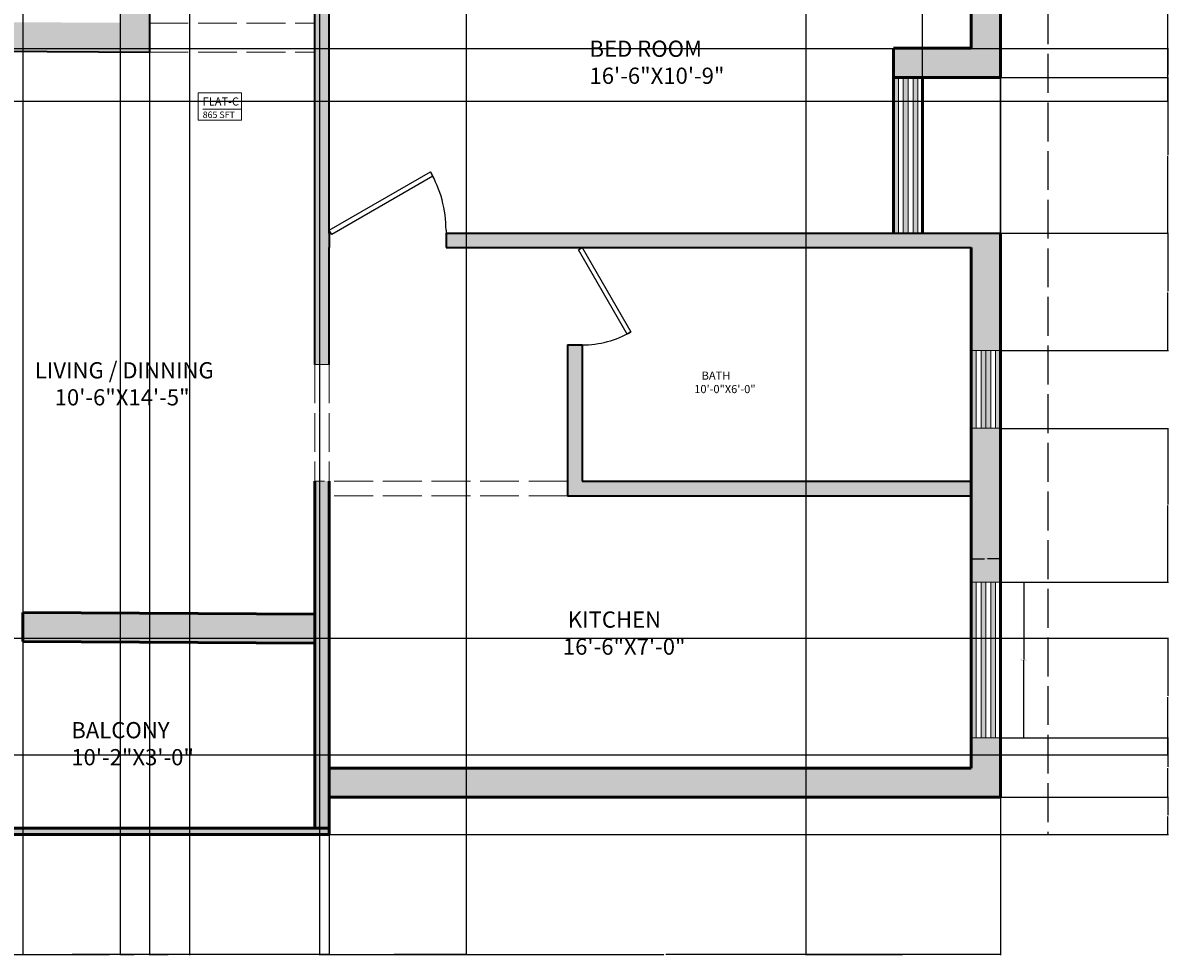
# Model space of a CAD drawing. Units: feet. Extents: x 2512 to 3087, y 1456 to 2266.
# Tile 2 of 5: x 2734 to 3087, y 1456 to 1744. Entities that reach past the tile are written whole.
import ezdxf

# ---------------------------------------------------------------- set-up
doc = ezdxf.new("R2010")
doc.units = ezdxf.units.FT
doc.linetypes.add('ACAD_ISO02W100', pattern=[15, 12, -3])
for name, color, linetype, lineweight in [('A-ANNO-DIMS', 2, 'Continuous', 18), ('A-AREA-IDEN', 7, 'Continuous', 18), ('A-DOOR', 240, 'Continuous', 25), ('A-GLAZ', 4, 'Continuous', 18), ('A-GLAZ-PATT', 252, 'Continuous', 13), ('A-WALL-OVHD', 8, 'ACAD_ISO02W100', 18), ('A-WALL-PATT', 252, 'Continuous', 13), ('ANNOTATION', 80, 'Continuous', 18), ('C-PROP', 8, 'ACAD_ISO02W100', 25), ('INNER WALL', 7, 'Continuous', 35), ('OPEN DOOR', 50, 'ACAD_ISO02W100', 18), ('OUTER WALL', 7, 'Continuous', 50)]:
    doc.layers.add(name, color=color, linetype=linetype, lineweight=lineweight)
doc.styles.get("Standard").update_dxf_attribs({"font": 'arial.ttf'})
doc.dimstyles.get("Standard").update_dxf_attribs({"dimtxt": 0.18, "dimasz": 0.18, "dimexe": 0.18, "dimexo": 0.0625, "dimgap": 0.09, "dimtad": 0, "dimtih": 1, "dimtoh": 1, "dimdec": 4, "dimzin": 0, "dimdsep": 46, "dimtxsty": 'Standard', "dimcen": 0.09, "dimadec": 0, "dimazin": 0, "dimtfac": 1, "dimtdec": 4, "dimtofl": 0, "dimtmove": 0, "dimatfit": 3, "dimfxl": 1, "dimtolj": 1, "dimtzin": 0, "dimarcsym": 0})

# ---------------------------------------------------------------- blocks, each defined once
blk = doc.blocks.new('*U7')
for p, q in [((0, 0), (0, -6)), ((40, 0), (40, -6))]:
    blk.add_line(p, q)
blk.add_lwpolyline([(0, 0), (34.64, 20), (35.52, 18.48), (0.87, -1.52)], close=True)
blk.add_arc((0, 0), 40, 0, 30)
blk = doc.blocks.new('WIN-48IN')
h = blk.add_hatch(color=256)
h.dxf.hatch_style = 1
h.paths.add_polyline_path([(0, 7.5), (0, 6), (48, 6), (48, 7.5)])
h.paths.add_polyline_path([(48, 3), (48, 4.5), (0, 4.5), (0, 3)])
h.paths.add_polyline_path([(48, 0), (48, 1.5), (0, 1.5), (0, 0)])
for p, q in [((0, 9), (48, 9)), ((0, 0), (0, 9)), ((0, 7.5), (48, 7.5)), ((48, 9), (48, 0)), ((0, 6), (48, 6)), ((0, 4.5), (48, 4.5)), ((0, 4.5), (48, 4.5)), ((0, 3), (48, 3)), ((0, 1.5), (48, 1.5)), ((48, 0), (0, 0))]:
    blk.add_line(p, q)
blk = doc.blocks.new('VENT-24IN')
h = blk.add_hatch(color=256)
h.dxf.hatch_style = 1
h.paths.add_polyline_path([(24, 7.5), (24, 9), (0, 9), (0, 7.5)])
h.paths.add_polyline_path([(0, 1.5), (0, 0), (24, 0), (24, 1.5)])
h.paths.add_polyline_path([(0, 4.5), (0, 3), (24, 3), (24, 4.5)])
h.paths.add_polyline_path([(24, 4.5), (24, 6), (0, 6), (0, 4.5)])
for p, q in [((0, 9), (24, 9)), ((0, 0), (0, 9)), ((0, 7.5), (24, 7.5)), ((24, 9), (24, 0)), ((0, 6), (24, 6)), ((0, 4.5), (24, 4.5)), ((0, 3), (24, 3)), ((0, 1.5), (24, 1.5)), ((24, 0), (0, 0))]:
    blk.add_line(p, q)
blk = doc.blocks.new('FLAT-ID-FRAME')
blk.add_line((1.44, 3.36), (13.18, 3.36))
blk.add_lwpolyline([(0, 8.39), (13.37, 8.39), (13.37, 0), (0, 0)], close=True)
blk = doc.blocks.new('*D13')
at = {"layer": 'A-ANNO-DIMS', "color": 0, "lineweight": -2, "transparency": 16777216}
for p, q in [((3035.28, 1571.08), (3042.6, 1571.08)), ((3042.42, 1570.9), (3042.42, 1547.26)), ((3042.42, 1523.26), (3042.42, 1546.89)), ((3035.28, 1523.08), (3042.6, 1523.08))]:
    blk.add_line(p, q, dxfattribs=at)
at = {"layer": 'A-ANNO-DIMS', "color": 0, "transparency": 16777216}
for points in [[(3042.39, 1570.9), (3042.45, 1570.9), (3042.42, 1571.08)], [(3042.39, 1523.26), (3042.45, 1523.26), (3042.42, 1523.08)]]:
    blk.add_solid(points, dxfattribs=at)
at = {"layer": 'Defpoints', "color": 0, "transparency": 16777216}
for p in [(3035.22, 1571.08), (3035.22, 1523.08), (3042.42, 1523.08)]:
    blk.add_point(p, dxfattribs=at)
at = {"layer": 'A-ANNO-DIMS', "color": 0, "transparency": 16777216, "insert": (3042.42, 1547.08), "char_height": 0.18, "attachment_point": 5}
blk.add_mtext('\\A1;WINDOW 48 TYP.', dxfattribs=at)
blk = doc.blocks.new('*D14')
at = {"layer": 'A-ANNO-DIMS', "color": 0, "lineweight": -2, "transparency": 16777216}
for p, q in [((3026.22, 1571.14), (3026.22, 1578.46)), ((3026.4, 1578.28), (3030.26, 1578.28)), ((3035.04, 1578.28), (3031.18, 1578.28)), ((3035.22, 1571.14), (3035.22, 1578.46))]:
    blk.add_line(p, q, dxfattribs=at)
at = {"layer": 'A-ANNO-DIMS', "color": 0, "transparency": 16777216}
for points in [[(3026.4, 1578.31), (3026.4, 1578.25), (3026.22, 1578.28)], [(3035.04, 1578.31), (3035.04, 1578.25), (3035.22, 1578.28)]]:
    blk.add_solid(points, dxfattribs=at)
at = {"layer": 'Defpoints', "color": 0, "transparency": 16777216}
for p in [(3035.22, 1578.28), (3026.22, 1571.08), (3035.22, 1571.08)]:
    blk.add_point(p, dxfattribs=at)
at = {"layer": 'A-ANNO-DIMS', "color": 0, "transparency": 16777216, "insert": (3030.72, 1578.28), "char_height": 0.18, "attachment_point": 5}
blk.add_mtext('\\A1;9 TYP.', dxfattribs=at)
blk = doc.blocks.new('*D23')
at = {"layer": 'A-ANNO-DIMS', "color": 0, "lineweight": -2, "transparency": 16777216}
for p, q in [((2772.72, 2204.17), (2772.72, 1456.05)), ((2785.14, 2204.17), (2785.14, 1456.05)), ((2772.9, 1456.23), (2778.48, 1456.23)), ((2784.96, 1456.23), (2779.38, 1456.23))]:
    blk.add_line(p, q, dxfattribs=at)
at = {"layer": 'A-ANNO-DIMS', "color": 0, "transparency": 16777216}
for points in [[(2772.9, 1456.26), (2772.9, 1456.2), (2772.72, 1456.23)], [(2784.96, 1456.26), (2784.96, 1456.2), (2785.14, 1456.23)]]:
    blk.add_solid(points, dxfattribs=at)
at = {"layer": 'Defpoints', "color": 0, "transparency": 16777216}
for p in [(2772.72, 2204.23), (2785.14, 2204.23), (2785.14, 1456.23)]:
    blk.add_point(p, dxfattribs=at)
at = {"layer": 'A-ANNO-DIMS', "color": 0, "transparency": 16777216, "insert": (2778.93, 1456.23), "char_height": 0.18, "attachment_point": 5}
blk.add_mtext('\\A1;12.422', dxfattribs=at)
blk = doc.blocks.new('*D24')
at = {"layer": 'A-ANNO-DIMS', "color": 0, "lineweight": -2, "transparency": 16777216}
for p, q in [((2825.22, 2204.17), (2825.22, 1456.05)), ((2870.39, 2204.17), (2870.39, 1456.05)), ((2825.4, 1456.23), (2847.41, 1456.23)), ((2870.21, 1456.23), (2848.2, 1456.23))]:
    blk.add_line(p, q, dxfattribs=at)
at = {"layer": 'A-ANNO-DIMS', "color": 0, "transparency": 16777216}
for points in [[(2825.4, 1456.26), (2825.4, 1456.2), (2825.22, 1456.23)], [(2870.21, 1456.26), (2870.21, 1456.2), (2870.39, 1456.23)]]:
    blk.add_solid(points, dxfattribs=at)
at = {"layer": 'Defpoints', "color": 0, "transparency": 16777216}
for p in [(2825.22, 2204.23), (2870.39, 2204.23), (2870.39, 1456.23)]:
    blk.add_point(p, dxfattribs=at)
at = {"layer": 'A-ANNO-DIMS', "color": 0, "transparency": 16777216, "insert": (2847.81, 1456.23), "char_height": 0.18, "attachment_point": 5}
blk.add_mtext('\\A1;45.17', dxfattribs=at)
blk = doc.blocks.new('*D27')
at = {"layer": 'A-ANNO-DIMS', "color": 0, "lineweight": -2, "transparency": 16777216}
for p, q in [((2693.22, 1493.17), (2693.22, 1456.05)), ((2828.22, 1493.17), (2828.22, 1456.05)), ((2693.4, 1456.23), (2760.44, 1456.23)), ((2828.04, 1456.23), (2761, 1456.23))]:
    blk.add_line(p, q, dxfattribs=at)
at = {"layer": 'A-ANNO-DIMS', "color": 0, "transparency": 16777216}
for points in [[(2693.4, 1456.26), (2693.4, 1456.2), (2693.22, 1456.23)], [(2828.04, 1456.26), (2828.04, 1456.2), (2828.22, 1456.23)]]:
    blk.add_solid(points, dxfattribs=at)
at = {"layer": 'Defpoints', "color": 0, "transparency": 16777216}
for p in [(2693.22, 1493.23), (2828.22, 1493.23), (2828.22, 1456.23)]:
    blk.add_point(p, dxfattribs=at)
at = {"layer": 'A-ANNO-DIMS', "color": 0, "transparency": 16777216, "insert": (2760.72, 1456.23), "char_height": 0.18, "attachment_point": 5}
blk.add_mtext('\\A1;135', dxfattribs=at)
blk = doc.blocks.new('*D28')
at = {"layer": 'A-ANNO-DIMS', "color": 0, "lineweight": -2, "transparency": 16777216}
for p, q in [((3035.22, 1504.67), (3035.22, 1456.05)), ((2828.22, 1493.17), (2828.22, 1456.05)), ((2828.4, 1456.23), (2931.43, 1456.23)), ((3035.04, 1456.23), (2932.01, 1456.23))]:
    blk.add_line(p, q, dxfattribs=at)
at = {"layer": 'A-ANNO-DIMS', "color": 0, "transparency": 16777216}
for points in [[(2828.4, 1456.26), (2828.4, 1456.2), (2828.22, 1456.23)], [(3035.04, 1456.26), (3035.04, 1456.2), (3035.22, 1456.23)]]:
    blk.add_solid(points, dxfattribs=at)
at = {"layer": 'Defpoints', "color": 0, "transparency": 16777216}
for p in [(3035.22, 1504.73), (2828.22, 1493.23), (3035.22, 1456.23)]:
    blk.add_point(p, dxfattribs=at)
at = {"layer": 'A-ANNO-DIMS', "color": 0, "transparency": 16777216, "insert": (2931.72, 1456.23), "char_height": 0.18, "attachment_point": 5}
blk.add_mtext('\\A1;207', dxfattribs=at)
blk = doc.blocks.new('*D30')
at = {"layer": 'A-ANNO-DIMS', "color": 0, "lineweight": -2, "transparency": 16777216}
for p, q in [((2633.28, 1553.8), (3087.03, 1553.8)), ((3086.85, 1553.62), (3086.85, 1535.98)), ((3086.85, 1517.98), (3086.85, 1535.62)), ((2633.28, 1517.8), (3087.03, 1517.8))]:
    blk.add_line(p, q, dxfattribs=at)
at = {"layer": 'A-ANNO-DIMS', "color": 0, "transparency": 16777216}
for points in [[(3086.82, 1553.62), (3086.88, 1553.62), (3086.85, 1553.8)], [(3086.82, 1517.98), (3086.88, 1517.98), (3086.85, 1517.8)]]:
    blk.add_solid(points, dxfattribs=at)
at = {"layer": 'Defpoints', "color": 0, "transparency": 16777216}
for p in [(2633.22, 1553.8), (3086.85, 1553.8), (2633.22, 1517.8)]:
    blk.add_point(p, dxfattribs=at)
at = {"layer": 'A-ANNO-DIMS', "color": 0, "transparency": 16777216, "insert": (3086.85, 1535.8), "char_height": 0.18, "attachment_point": 5}
blk.add_mtext('\\A1;36', dxfattribs=at)
blk = doc.blocks.new('*D32')
at = {"layer": 'A-ANNO-DIMS', "color": 0, "lineweight": -2, "transparency": 16777216}
for p, q in [((2828.28, 1504.73), (3087.03, 1504.73)), ((3086.85, 1504.55), (3086.85, 1499.16)), ((3086.85, 1493.41), (3086.85, 1498.8)), ((2828.28, 1493.23), (3087.03, 1493.23))]:
    blk.add_line(p, q, dxfattribs=at)
at = {"layer": 'A-ANNO-DIMS', "color": 0, "transparency": 16777216}
for points in [[(3086.82, 1504.55), (3086.88, 1504.55), (3086.85, 1504.73)], [(3086.82, 1493.41), (3086.88, 1493.41), (3086.85, 1493.23)]]:
    blk.add_solid(points, dxfattribs=at)
at = {"layer": 'Defpoints', "color": 0, "transparency": 16777216}
for p in [(2828.22, 1504.73), (3086.85, 1504.73), (2828.22, 1493.23)]:
    blk.add_point(p, dxfattribs=at)
at = {"layer": 'A-ANNO-DIMS', "color": 0, "transparency": 16777216, "insert": (3086.85, 1498.98), "char_height": 0.18, "attachment_point": 5}
blk.add_mtext('\\A1;11.5', dxfattribs=at)
blk = doc.blocks.new('*D33')
at = {"layer": 'A-ANNO-DIMS', "color": 0, "lineweight": -2, "transparency": 16777216}
for p, q in [((3035.28, 1523.08), (3087.03, 1523.08)), ((3086.85, 1522.9), (3086.85, 1514.09)), ((3086.85, 1504.91), (3086.85, 1513.72)), ((3035.28, 1504.73), (3087.03, 1504.73))]:
    blk.add_line(p, q, dxfattribs=at)
at = {"layer": 'A-ANNO-DIMS', "color": 0, "transparency": 16777216}
for points in [[(3086.82, 1522.9), (3086.88, 1522.9), (3086.85, 1523.08)], [(3086.82, 1504.91), (3086.88, 1504.91), (3086.85, 1504.73)]]:
    blk.add_solid(points, dxfattribs=at)
at = {"layer": 'Defpoints', "color": 0, "transparency": 16777216}
for p in [(3035.22, 1523.08), (3086.85, 1523.08), (3035.22, 1504.73)]:
    blk.add_point(p, dxfattribs=at)
at = {"layer": 'A-ANNO-DIMS', "color": 0, "transparency": 16777216, "insert": (3086.85, 1513.9), "char_height": 0.18, "attachment_point": 5}
blk.add_mtext('\\A1;18.345', dxfattribs=at)
blk = doc.blocks.new('*D34')
at = {"layer": 'A-ANNO-DIMS', "color": 0, "lineweight": -2, "transparency": 16777216}
for p, q in [((3035.28, 1618.51), (3087.03, 1618.51)), ((3086.85, 1618.33), (3086.85, 1594.97)), ((3086.85, 1571.26), (3086.85, 1594.61)), ((3035.28, 1571.08), (3087.03, 1571.08))]:
    blk.add_line(p, q, dxfattribs=at)
at = {"layer": 'A-ANNO-DIMS', "color": 0, "transparency": 16777216}
for points in [[(3086.82, 1618.33), (3086.88, 1618.33), (3086.85, 1618.51)], [(3086.82, 1571.26), (3086.88, 1571.26), (3086.85, 1571.08)]]:
    blk.add_solid(points, dxfattribs=at)
at = {"layer": 'Defpoints', "color": 0, "transparency": 16777216}
for p in [(3035.22, 1618.51), (3086.85, 1618.51), (3035.22, 1571.08)]:
    blk.add_point(p, dxfattribs=at)
at = {"layer": 'A-ANNO-DIMS', "color": 0, "transparency": 16777216, "insert": (3086.85, 1594.79), "char_height": 0.18, "attachment_point": 5}
blk.add_mtext('\\A1;47.44', dxfattribs=at)
blk = doc.blocks.new('*D35')
at = {"layer": 'A-ANNO-DIMS', "color": 0, "lineweight": -2, "transparency": 16777216}
for p, q in [((3035.28, 1678.73), (3087.03, 1678.73)), ((3086.85, 1678.55), (3086.85, 1660.8)), ((3086.85, 1642.69), (3086.85, 1660.44)), ((3035.28, 1642.51), (3087.03, 1642.51))]:
    blk.add_line(p, q, dxfattribs=at)
at = {"layer": 'A-ANNO-DIMS', "color": 0, "transparency": 16777216}
for points in [[(3086.82, 1678.55), (3086.88, 1678.55), (3086.85, 1678.73)], [(3086.82, 1642.69), (3086.88, 1642.69), (3086.85, 1642.51)]]:
    blk.add_solid(points, dxfattribs=at)
at = {"layer": 'Defpoints', "color": 0, "transparency": 16777216}
for p in [(3035.22, 1678.73), (3086.85, 1678.73), (3035.22, 1642.51)]:
    blk.add_point(p, dxfattribs=at)
at = {"layer": 'A-ANNO-DIMS', "color": 0, "transparency": 16777216, "insert": (3086.85, 1660.62), "char_height": 0.18, "attachment_point": 5}
blk.add_mtext('\\A1;36.22', dxfattribs=at)
blk = doc.blocks.new('*D36')
at = {"layer": 'A-ANNO-DIMS', "color": 0, "lineweight": -2, "transparency": 16777216}
for p, q in [((3035.28, 1726.73), (3087.03, 1726.73)), ((3086.85, 1726.55), (3086.85, 1702.91)), ((3086.85, 1678.91), (3086.85, 1702.55)), ((3035.28, 1678.73), (3087.03, 1678.73))]:
    blk.add_line(p, q, dxfattribs=at)
at = {"layer": 'A-ANNO-DIMS', "color": 0, "transparency": 16777216}
for points in [[(3086.82, 1726.55), (3086.88, 1726.55), (3086.85, 1726.73)], [(3086.82, 1678.91), (3086.88, 1678.91), (3086.85, 1678.73)]]:
    blk.add_solid(points, dxfattribs=at)
at = {"layer": 'Defpoints', "color": 0, "transparency": 16777216}
for p in [(3035.22, 1726.73), (3086.85, 1726.73), (3035.22, 1678.73)]:
    blk.add_point(p, dxfattribs=at)
at = {"layer": 'A-ANNO-DIMS', "color": 0, "transparency": 16777216, "insert": (3086.85, 1702.73), "char_height": 0.18, "attachment_point": 5}
blk.add_mtext('\\A1;48', dxfattribs=at)
blk = doc.blocks.new('*D37')
at = {"layer": 'A-ANNO-DIMS', "color": 0, "lineweight": -2, "transparency": 16777216}
for p, q in [((3026.28, 1816.73), (3087.03, 1816.73)), ((3086.85, 1816.55), (3086.85, 1771.91)), ((3086.85, 1726.91), (3086.85, 1771.55)), ((3035.28, 1726.73), (3087.03, 1726.73))]:
    blk.add_line(p, q, dxfattribs=at)
at = {"layer": 'A-ANNO-DIMS', "color": 0, "transparency": 16777216}
for points in [[(3086.82, 1816.55), (3086.88, 1816.55), (3086.85, 1816.73)], [(3086.82, 1726.91), (3086.88, 1726.91), (3086.85, 1726.73)]]:
    blk.add_solid(points, dxfattribs=at)
at = {"layer": 'Defpoints', "color": 0, "transparency": 16777216}
for p in [(3026.22, 1816.73), (3086.85, 1816.73), (3035.22, 1726.73)]:
    blk.add_point(p, dxfattribs=at)
at = {"layer": 'A-ANNO-DIMS', "color": 0, "transparency": 16777216, "insert": (3086.85, 1771.73), "char_height": 0.18, "attachment_point": 5}
blk.add_mtext('\\A1;90', dxfattribs=at)
blk = doc.blocks.new('*D44')
at = {"layer": 'A-ANNO-DIMS', "color": 0, "lineweight": -2, "transparency": 16777216}
for p, q in [((2975.22, 2135.17), (2975.22, 1456.05)), ((3035.22, 2135.17), (3035.22, 1456.05)), ((2975.4, 1456.23), (3005, 1456.23)), ((3035.04, 1456.23), (3005.44, 1456.23))]:
    blk.add_line(p, q, dxfattribs=at)
at = {"layer": 'A-ANNO-DIMS', "color": 0, "transparency": 16777216}
for points in [[(2975.4, 1456.26), (2975.4, 1456.2), (2975.22, 1456.23)], [(3035.04, 1456.26), (3035.04, 1456.2), (3035.22, 1456.23)]]:
    blk.add_solid(points, dxfattribs=at)
at = {"layer": 'Defpoints', "color": 0, "transparency": 16777216}
for p in [(2975.22, 2135.23), (3035.22, 2135.23), (3035.22, 1456.23)]:
    blk.add_point(p, dxfattribs=at)
at = {"layer": 'A-ANNO-DIMS', "color": 0, "transparency": 16777216, "insert": (3005.22, 1456.23), "char_height": 0.18, "attachment_point": 5}
blk.add_mtext('\\A1;60', dxfattribs=at)
blk = doc.blocks.new('*D45')
at = {"layer": 'A-ANNO-DIMS', "color": 0, "lineweight": -2, "transparency": 16777216}
for p, q in [((3011.22, 1678.79), (3011.22, 2266.2)), ((3011.4, 2266.02), (3023, 2266.02)), ((3035.04, 2266.02), (3023.44, 2266.02)), ((3035.22, 1678.79), (3035.22, 2266.2))]:
    blk.add_line(p, q, dxfattribs=at)
at = {"layer": 'A-ANNO-DIMS', "color": 0, "transparency": 16777216}
for points in [[(3011.4, 2266.05), (3011.4, 2265.99), (3011.22, 2266.02)], [(3035.04, 2266.05), (3035.04, 2265.99), (3035.22, 2266.02)]]:
    blk.add_solid(points, dxfattribs=at)
at = {"layer": 'Defpoints', "color": 0, "transparency": 16777216}
for p in [(3035.22, 2266.02), (3011.22, 1678.73), (3035.22, 1678.73)]:
    blk.add_point(p, dxfattribs=at)
at = {"layer": 'A-ANNO-DIMS', "color": 0, "transparency": 16777216, "insert": (3023.22, 2266.02), "char_height": 0.18, "attachment_point": 5}
blk.add_mtext('\\A1;24', dxfattribs=at)
blk = doc.blocks.new('*D49')
at = {"layer": 'A-ANNO-DIMS', "color": 0, "lineweight": -2, "transparency": 16777216}
for p, q in [((2573.28, 1735.68), (3087.03, 1735.68)), ((3086.85, 1735.5), (3086.85, 1727.7)), ((3086.85, 1719.55), (3086.85, 1727.34)), ((2573.28, 1719.37), (3087.03, 1719.37))]:
    blk.add_line(p, q, dxfattribs=at)
at = {"layer": 'A-ANNO-DIMS', "color": 0, "transparency": 16777216}
for points in [[(3086.82, 1735.5), (3086.88, 1735.5), (3086.85, 1735.68)], [(3086.82, 1719.55), (3086.88, 1719.55), (3086.85, 1719.37)]]:
    blk.add_solid(points, dxfattribs=at)
at = {"layer": 'Defpoints', "color": 0, "transparency": 16777216}
for p in [(2573.22, 1735.68), (3086.85, 1735.68), (2573.22, 1719.37)]:
    blk.add_point(p, dxfattribs=at)
at = {"layer": 'A-ANNO-DIMS', "color": 0, "transparency": 16777216, "insert": (3086.85, 1727.52), "char_height": 0.18, "attachment_point": 5}
blk.add_mtext('\\A1;16.305', dxfattribs=at)
blk = doc.blocks.new('*D53')
at = {"layer": 'A-ANNO-DIMS', "color": 0, "lineweight": -2, "transparency": 16777216}
for p, q in [((2733.72, 2127.67), (2733.72, 1456.05)), ((2763.72, 2127.67), (2763.72, 1456.05)), ((2733.9, 1456.23), (2748.5, 1456.23)), ((2763.54, 1456.23), (2748.94, 1456.23))]:
    blk.add_line(p, q, dxfattribs=at)
at = {"layer": 'A-ANNO-DIMS', "color": 0, "transparency": 16777216}
for points in [[(2733.9, 1456.26), (2733.9, 1456.2), (2733.72, 1456.23)], [(2763.54, 1456.26), (2763.54, 1456.2), (2763.72, 1456.23)]]:
    blk.add_solid(points, dxfattribs=at)
at = {"layer": 'Defpoints', "color": 0, "transparency": 16777216}
for p in [(2733.72, 2127.73), (2763.72, 2127.73), (2763.72, 1456.23)]:
    blk.add_point(p, dxfattribs=at)
at = {"layer": 'A-ANNO-DIMS', "color": 0, "transparency": 16777216, "insert": (2748.72, 1456.23), "char_height": 0.18, "attachment_point": 5}
blk.add_mtext('\\A1;30', dxfattribs=at)
blk = doc.blocks.new('*D54')
at = {"layer": 'A-ANNO-DIMS', "color": 0, "lineweight": -2, "transparency": 16777216}
for p, q in [((2772.72, 2132.17), (2772.72, 1456.05)), ((2763.72, 2127.67), (2763.72, 1456.05)), ((2763.9, 1456.23), (2768.07, 1456.23)), ((2772.54, 1456.23), (2768.37, 1456.23))]:
    blk.add_line(p, q, dxfattribs=at)
at = {"layer": 'A-ANNO-DIMS', "color": 0, "transparency": 16777216}
for points in [[(2763.9, 1456.26), (2763.9, 1456.2), (2763.72, 1456.23)], [(2772.54, 1456.26), (2772.54, 1456.2), (2772.72, 1456.23)]]:
    blk.add_solid(points, dxfattribs=at)
at = {"layer": 'Defpoints', "color": 0, "transparency": 16777216}
for p in [(2772.72, 2132.23), (2763.72, 2127.73), (2772.72, 1456.23)]:
    blk.add_point(p, dxfattribs=at)
at = {"layer": 'A-ANNO-DIMS', "color": 0, "transparency": 16777216, "insert": (2768.22, 1456.23), "char_height": 0.18, "attachment_point": 5}
blk.add_mtext('\\A1;9', dxfattribs=at)

msp = doc.modelspace()

# ---------------------------------------------------------------- hatches: boundary and pattern name
at = {"layer": 'A-GLAZ-PATT'}
h = msp.add_hatch(color=256, dxfattribs=at)
h.dxf.hatch_style = 1
h.paths.add_polyline_path([(3009.7546, 1726.7316), (3008.2546, 1726.7316), (3008.2546, 1678.7316), (3009.7546, 1678.7316)])
h.paths.add_polyline_path([(3005.2546, 1678.7316), (3006.7546, 1678.7316), (3006.7546, 1726.7316), (3005.2546, 1726.7316)])
h.paths.add_polyline_path([(3002.2546, 1678.7316), (3003.7546, 1678.7316), (3003.7546, 1726.7316), (3002.2546, 1726.7316)])
at = {"layer": 'A-WALL-PATT'}
h = msp.add_hatch(color=256, dxfattribs=at)
h.dxf.hatch_style = 1
h.paths.add_polyline_path([(3035.2185, 1915.2872), (3026.2185, 1915.2872), (3026.2185, 1912.7316), (2936.2185, 1912.7316), (2936.2185, 2001.7316), (2931.7185, 2001.7316), (2931.7185, 1912.7316), (2808.7185, 1912.7316), (2808.7185, 1903.7316), (3026.2185, 1903.7316), (3026.2185, 1816.7316), (2808.7185, 1816.7316), (2808.7185, 1807.7316), (2823.7185, 1807.7316), (2823.7185, 1638.2316), (2828.2185, 1638.2316), (2828.2185, 1674.2316), (2828.2185, 1678.7316), (2828.2185, 1807.7316), (3026.2185, 1807.7316), (3026.2185, 1735.7316), (3002.2185, 1735.7316), (3002.2546, 1726.7316), (3011.2546, 1726.7316), (3035.2185, 1726.7316)])
h.paths.add_polyline_path([(3035.2185, 2001.7316), (2990.2185, 2001.7316), (2972.2185, 2001.7316), (2972.2185, 1996.7316), (3026.2185, 1996.7316), (3026.2185, 1963.2872), (3035.2185, 1963.2872)], flags=17)
h.paths.add_polyline_path([(3041.2185, 2010.7316), (2990.2185, 2010.7316), (2990.2185, 2001.7316), (3035.2185, 2001.7316), (3041.2185, 2001.7316)])
h.paths.add_polyline_path([(3044.2185, 2085.7316), (3044.2185, 2088.2316), (3041.2185, 2088.2316), (3041.2185, 2006.2316), (3044.2185, 2006.2316)])
h.paths.add_polyline_path([(3041.2185, 2090.2316), (2975.2185, 2090.2316), (2975.2185, 2090.2254), (2966.2185, 2090.2254), (2825.2185, 2090.2316), (2825.2185, 2091.7316), (2820.7185, 2091.7316), (2820.7185, 2085.7316), (2820.7185, 2084.2316), (2825.2185, 2084.2316), (2825.2185, 2085.7316), (2990.2185, 2085.7316), (2990.2185, 2046.7316), (2999.2185, 2046.7316), (2999.2185, 2085.7316), (3041.2185, 2085.7316)])
h.paths.add_polyline_path([(3035.2185, 2213.2316), (2918.3922, 2213.2316), (2918.3922, 2204.2316), (3026.2185, 2204.2316), (3026.2185, 2144.2316), (2966.2185, 2144.2316), (2966.2185, 2135.213), (2975.2185, 2135.213), (2975.2185, 2135.2316), (3035.2185, 2135.2316)])
h.paths.add_polyline_path([(2870.3922, 2213.2316), (2809.1404, 2213.2316), (2809.1404, 2204.2316), (2820.7185, 2204.2316), (2820.7185, 2162.2316), (2825.2185, 2162.2316), (2825.2185, 2204.2316), (2870.3922, 2204.2316)])
h.paths.add_polyline_path([(2785.1404, 2213.2316), (2751.447, 2213.2316), (2751.447, 2204.2316), (2763.7185, 2204.2316), (2763.7185, 2127.7316), (2825.2185, 2127.7316), (2825.2185, 2132.2316), (2820.7185, 2132.2316), (2772.7185, 2132.2316), (2772.7185, 2204.2316), (2785.1404, 2204.2316)])
h.paths.add_polyline_path([(2727.447, 2213.2316), (2656.8898, 2213.2316), (2656.8898, 2204.2316), (2711.2185, 2204.2316), (2711.2185, 2124.7316), (2715.7185, 2124.7316), (2715.7185, 2127.7316), (2733.7185, 2127.7316), (2733.7185, 2132.2316), (2715.7185, 2132.2316), (2715.7185, 2204.2316), (2727.447, 2204.2316)], flags=17)
h.paths.add_polyline_path([(2608.8898, 2213.2316), (2564.2185, 2213.2316), (2564.2185, 2079.7316), (2609.2185, 2079.7316), (2609.2185, 2037.7316), (2618.2185, 2037.7316), (2618.2185, 2079.7316), (2763.7185, 2079.7316), (2763.7185, 2007.7316), (2654.2185, 2007.7316), (2654.2185, 2003.2316), (2763.7185, 2003.2316), (2763.7185, 1891.0755), (2772.7185, 1891.0234), (2772.7185, 1903.7316), (2772.7185, 2088.7316), (2573.2185, 2088.7316), (2573.2185, 2204.2316), (2608.8898, 2204.2316)])
h.paths.add_polyline_path([(2567.2185, 2079.7316), (2564.2185, 2079.7316), (2564.2185, 2007.7316), (2567.2185, 2007.7316)], flags=17)
h.paths.add_polyline_path([(2618.2185, 2007.7316), (2564.2185, 2007.7316), (2564.2185, 2003.2171), (2573.2185, 2003.2171), (2573.2185, 2003.2316), (2618.2185, 2003.2316)], flags=17)
h.paths.add_polyline_path([(2573.2185, 1955.2171), (2564.2185, 1955.2171), (2564.2185, 1904.096), (2573.2185, 1904.096)], flags=17)
h.paths.add_polyline_path([(2573.2185, 1851.677), (2603.2185, 1851.5035), (2603.2195, 1856.0035), (2573.2185, 1856.1771), (2573.2185, 1856.096), (2564.2185, 1856.096), (2564.2185, 1785.728), (2594.2185, 1785.5544), (2600.2185, 1785.5197), (2637.7185, 1785.3028), (2637.7185, 1855.8039), (2633.2185, 1855.83), (2633.2185, 1789.8289), (2573.2185, 1790.176)])
h.paths.add_polyline_path([(2772.7185, 1855.0228), (2767.3185, 1855.0228), (2767.3004, 1855.0542), (2673.7185, 1855.5956), (2673.7185, 1851.0956), (2763.7185, 1850.575), (2763.7185, 1743.5732), (2564.2185, 1744.7273), (2564.2185, 1719.3701), (2573.2185, 1719.3701), (2573.2185, 1735.6751), (2633.2185, 1735.328), (2633.2185, 1717.3272), (2637.7185, 1717.3272), (2637.7185, 1735.302), (2772.7185, 1734.521)])
h.paths.add_polyline_path([(2697.7185, 1734.9549), (2693.2185, 1734.9809), (2693.2185, 1602.8011), (2697.7185, 1602.8011)])
h.paths.add_polyline_path([(2823.7185, 1561.2231), (2733.7185, 1561.7437), (2733.7185, 1552.7436), (2823.7185, 1552.2229)])
h.paths.add_polyline_path([(2697.7185, 1566.8011), (2693.2185, 1566.8011), (2693.2185, 1562.8011), (2682.4194, 1562.8011), (2682.4194, 1553.8011), (2693.2185, 1553.8011), (2693.2185, 1495.2316), (2697.7185, 1495.2316)])
h.paths.add_polyline_path([(2828.2185, 1495.2316), (2693.2185, 1495.2316), (2693.2185, 1493.2316), (2828.2185, 1493.2316)])
h.paths.add_polyline_path([(2828.2185, 1602.2316), (2823.7185, 1602.2316), (2823.7185, 1495.2316), (2828.2185, 1495.2316)])
h.paths.add_polyline_path([(3035.2185, 1523.0765), (3026.2185, 1523.0765), (3026.2185, 1513.7316), (2828.2185, 1513.7316), (2828.2185, 1504.7316), (3035.2185, 1504.7316)])
h.paths.add_polyline_path([(3026.2185, 1602.2316), (2906.2185, 1602.2316), (2906.2185, 1644.2316), (2901.7185, 1644.2316), (2901.7185, 1597.7316), (3026.2185, 1597.7316)])
h.paths.add_polyline_path([(3035.2185, 1678.7316), (2864.2185, 1678.7316), (2864.2185, 1674.2316), (3026.2185, 1674.2316), (3026.2185, 1642.5123), (3035.2185, 1642.5123)], flags=17)
h.paths.add_polyline_path([(3035.2185, 1618.5123), (3026.2185, 1618.5123), (3026.2185, 1571.0765), (3035.2185, 1571.0765)])
h = msp.add_hatch(color=256, dxfattribs=at)
h.dxf.hatch_style = 1
h.paths.add_polyline_path([(2573.2185, 1683.1742), (2637.6925, 1682.8012), (2637.6947, 1687.3013), (2573.2185, 1687.6743), (2573.2185, 1695.3702), (2564.2185, 1695.3702), (2564.2185, 1517.8011), (2624.2185, 1517.8011), (2633.2185, 1517.8011), (2633.2185, 1553.8011), (2634.4194, 1553.8011), (2634.4194, 1562.8011), (2624.2185, 1562.8011), (2624.2185, 1526.8011), (2573.2185, 1526.8011)])
h.paths.add_polyline_path([(2573.2185, 1735.6751), (2633.2185, 1735.328), (2633.2185, 1717.3272), (2637.7096, 1717.3272), (2637.7185, 1735.302), (2772.7185, 1734.521), (2772.7185, 1855.0228), (2673.7185, 1855.5956), (2673.7185, 1851.0956), (2763.7185, 1850.575), (2763.7185, 1743.5732), (2564.2185, 1744.7273), (2564.2185, 1719.3701), (2573.2185, 1719.3701)])
h.paths.add_polyline_path([(2828.2185, 1807.7316), (3026.2185, 1807.7316), (3026.2185, 1735.7316), (3002.2185, 1735.7316), (3002.2546, 1726.7316), (3011.2546, 1726.7316), (3035.2185, 1726.7316), (3035.2185, 1915.2872), (3026.2185, 1915.2872), (3026.2185, 1912.7316), (2936.2185, 1912.7316), (2936.2185, 2001.7316), (2931.7185, 2001.7316), (2931.7185, 1912.7316), (2808.7185, 1912.7316), (2808.7185, 1903.7316), (3026.2185, 1903.7316), (3026.2185, 1816.7316), (2808.7185, 1816.7316), (2808.7185, 1807.7316), (2823.7185, 1807.7316), (2823.7185, 1638.2316), (2828.2185, 1638.2316), (2828.2185, 1674.2316), (2828.2185, 1678.7316)])
h.paths.add_polyline_path([(3035.2185, 1678.7316), (2864.2185, 1678.7316), (2864.2185, 1674.2316), (3026.2185, 1674.2316), (3026.2185, 1642.5123), (3035.2185, 1642.5123)], flags=17)
h.paths.add_polyline_path([(3035.2185, 1618.5123), (3026.2185, 1618.5123), (3026.2185, 1571.0765), (3035.2185, 1571.0765)])
h.paths.add_polyline_path([(3026.2185, 1602.2316), (2906.2185, 1602.2316), (2906.2185, 1644.2316), (2901.7185, 1644.2316), (2901.7185, 1597.7316), (3026.2185, 1597.7316)])
h.paths.add_polyline_path([(3035.2185, 1523.0765), (3026.2185, 1523.0765), (3026.2185, 1513.7316), (2828.2185, 1513.7316), (2828.2185, 1504.7316), (3035.2185, 1504.7316)])
h.paths.add_polyline_path([(2828.2185, 1495.2316), (2693.2185, 1495.2316), (2693.2185, 1493.2316), (2828.2185, 1493.2316)])
h.paths.add_polyline_path([(2828.2185, 1602.2316), (2823.7185, 1602.2316), (2823.7185, 1495.2316), (2828.2185, 1495.2316)])
h.paths.add_polyline_path([(2823.7185, 1561.2231), (2733.7185, 1561.7437), (2733.7185, 1552.7436), (2823.7185, 1552.2229)])
h.paths.add_polyline_path([(2697.7185, 1566.8011), (2693.2185, 1566.8011), (2693.2185, 1562.8011), (2682.4194, 1562.8011), (2682.4194, 1553.8011), (2693.2185, 1553.8011), (2693.2185, 1495.2316), (2697.7185, 1495.2316)])
h.paths.add_polyline_path([(2697.7185, 1734.9549), (2693.2185, 1734.9809), (2693.2185, 1602.8011), (2697.7185, 1602.8011)])
h.paths.add_polyline_path([(2573.2185, 1851.677), (2603.2185, 1851.5035), (2603.2195, 1856.0035), (2573.2185, 1856.1771), (2573.2185, 1856.096), (2564.2185, 1856.096), (2564.2185, 1785.728), (2594.2185, 1785.5544), (2600.2185, 1785.5197), (2637.7185, 1785.3028), (2637.7185, 1855.8039), (2633.2185, 1855.83), (2633.2185, 1789.8289), (2573.2185, 1790.176)])
h.paths.add_polyline_path([(2573.2185, 1955.2171), (2564.2185, 1955.2171), (2564.2185, 1904.096), (2573.2185, 1904.096)])
h.paths.add_polyline_path([(2618.2185, 2007.7316), (2564.2185, 2007.7316), (2564.2185, 2003.2171), (2573.2185, 2003.2171), (2573.2185, 2003.2316), (2618.2185, 2003.2316)])
h.paths.add_polyline_path([(2567.2185, 2079.7316), (2564.2185, 2079.7316), (2564.2185, 2007.7316), (2567.2185, 2007.7316)])

# ---------------------------------------------------------------- linework, layer by layer
at = {"layer": 'A-GLAZ'}
for p, q in [((3002.2546, 1678.7316), (3002.2546, 1726.7316)), ((3002.2546, 1726.7316), (3011.2546, 1726.7316)), ((3003.7546, 1726.7316), (3003.7546, 1678.7316)), ((3005.2546, 1726.7316), (3005.2546, 1678.7316)), ((3006.7546, 1726.7316), (3006.7546, 1678.7316)), ((3006.7546, 1726.7316), (3006.7546, 1678.7316)), ((3008.2546, 1726.7316), (3008.2546, 1678.7316)), ((3009.7546, 1726.7316), (3009.7546, 1678.7316)), ((3011.2546, 1726.7316), (3011.2546, 1678.7316)), ((3011.2546, 1678.7316), (3002.2546, 1678.7316))]:
    msp.add_line(p, q, dxfattribs=at)
at = {"layer": 'A-WALL-OVHD'}
msp.add_line((3035.2185, 1726.7316), (3035.2185, 1678.7316), dxfattribs=at)
at = {"layer": 'C-PROP'}
for p in [(3049.8469, 2229.0217), (2828.2185, 1493.2316)]:
    msp.add_line(p, (3049.8469, 1493.2316), dxfattribs=at)
at = {"layer": 'INNER WALL'}
for p, q in [((2772.7185, 1855.0228), (2772.7185, 1734.521)), ((2823.7185, 1638.2316), (2823.7185, 1807.7316)), ((2828.2185, 1678.7316), (2828.2185, 1807.7316)), ((2637.7185, 1735.302), (2772.7185, 1734.521)), ((2828.2185, 1678.7316), (2828.2185, 1674.2316)), ((2864.2185, 1678.7316), (3035.2185, 1678.7316)), ((2864.2185, 1678.7316), (2864.2185, 1674.2316)), ((2828.2185, 1638.2316), (2828.2185, 1674.2316)), ((2864.2185, 1674.2316), (3026.2185, 1674.2316)), ((2901.7185, 1644.2316), (2901.7185, 1597.7316)), ((2901.7185, 1644.2316), (2906.2185, 1644.2316)), ((2906.2185, 1644.2316), (2906.2185, 1602.2316)), ((2906.2185, 1644.2316), (2906.2185, 1602.2316)), ((2906.2185, 1602.2316), (3026.2185, 1602.2316)), ((2901.7185, 1597.7316), (3026.2185, 1597.7316))]:
    msp.add_line(p, q, dxfattribs=at)
at = {"layer": 'OPEN DOOR'}
for p, q in [((2772.7185, 1743.521), (2823.7185, 1743.521)), ((2772.7185, 1734.521), (2823.7185, 1734.521)), ((2828.2185, 1638.2316), (2823.7185, 1638.2316)), ((2823.7185, 1638.2316), (2823.7185, 1602.2316)), ((2828.2185, 1638.2316), (2828.2185, 1602.2316)), ((2901.7185, 1602.2316), (2823.7185, 1602.2316)), ((2901.7185, 1597.7316), (2828.2185, 1597.7316))]:
    msp.add_line(p, q, dxfattribs=at)
at = {"layer": 'OUTER WALL'}
for p, q in [((3035.2185, 2001.7316), (3035.2185, 1726.7316)), ((3026.2185, 1807.7316), (3026.2185, 1735.7316)), ((3026.2185, 1735.7316), (3002.2185, 1735.7316)), ((3002.2546, 1726.7316), (3002.2185, 1735.7316)), ((3035.2185, 1726.7316), (3002.2185, 1726.7316)), ((3002.2185, 1726.7316), (3002.2185, 1678.7316)), ((3011.2185, 1726.7316), (3011.2185, 1678.7316)), ((3035.2185, 1678.7316), (3035.2185, 1504.7316)), ((3026.2185, 1674.2316), (3026.2185, 1513.7316)), ((2823.7185, 1495.2316), (2823.7185, 1602.2316)), ((2828.2185, 1493.2316), (2828.2185, 1602.2316)), ((2733.7185, 1561.7437), (2823.7185, 1561.2231)), ((2733.7185, 1552.7436), (2733.7185, 1561.7437)), ((2733.7185, 1552.7436), (2823.6664, 1552.2232)), ((2828.2185, 1513.7316), (3026.2185, 1513.7316)), ((2828.2185, 1504.7316), (3035.2185, 1504.7316)), ((2828.2185, 1495.2316), (2693.2185, 1495.2316)), ((2693.2185, 1493.2316), (2828.2185, 1493.2316))]:
    msp.add_line(p, q, dxfattribs=at)

# ---------------------------------------------------------------- block references
at = {"layer": 'A-AREA-IDEN'}
msp.add_blockref('FLAT-ID-FRAME', (2787.7182, 1713.6012), dxfattribs=at)
at = {"layer": 'A-DOOR', "xscale": 0.899999999999959, "yscale": 0.899999999999959, "zscale": 0.899999999999959}
msp.add_blockref('*U7', (2828.2185, 1679.6316), dxfattribs=at)
at = {"layer": 'A-DOOR', "xscale": 0.7500000000000038, "yscale": 0.7500000000000038, "zscale": 0.7500000000000038, "rotation": 270}
msp.add_blockref('*U7', (2906.2185, 1674.2316), dxfattribs=at)
at = {"layer": 'A-GLAZ'}
for name, p, rotation in [('VENT-24IN', (3026.2189, 1642.5123), 269.9999999999984), ('WIN-48IN', (3026.2189, 1571.0763), 269.9999999999929)]:
    msp.add_blockref(name, p, dxfattribs=dict(at, rotation=rotation))

# ---------------------------------------------------------------- texts
at = {"layer": 'A-AREA-IDEN', "attachment_point": 1}
for s, width, insert, char_height in [('FLAT-C', 12.525641, (2789.1599, 1720.5613), 2.5), ('865 SFT', 11.390914, (2789.1599, 1716.2188), 2)]:
    msp.add_mtext_dynamic_manual_height_columns(s, width=width, gutter_width=12.5, heights=[0], dxfattribs=dict(at, insert=insert, char_height=char_height))
at = {"layer": 'ANNOTATION', "attachment_point": 1}
for s, width, insert, char_height in [('\\A1;BED ROOM\\P16\'-6"X10\'-9"', 38.558323, (2908.4638, 1738.0911), 5), ('\\A1;LIVING / DINNING\\P    10\'-6"X14\'-5"', 59.172495, (2737.3929, 1638.9154), 5), ('   BATH\\P10\'-0"X6\'-0"', 16.842597, (2940.7704, 1636.0297), 2.5), ('\\A1; KITCHEN\\P16\'-6"X7\'-0"', 38.558323, (2900.251, 1562.028), 5), ('\\A1;BALCONY\\P10\'-2"X3\'-0"', 38.558323, (2748.6345, 1527.9183), 5)]:
    msp.add_mtext_dynamic_manual_height_columns(s, width=width, gutter_width=12.5, heights=[0], dxfattribs=dict(at, insert=insert, char_height=char_height))

# ---------------------------------------------------------------- dimensions: what is measured, and where the dimension line sits
at = {"layer": 'A-ANNO-DIMS'}
for base, p1, p2, override, picture, middle in [((3035.2185, 2266.0217), (3011.2185, 1678.7316), (3035.2185, 1678.7316), {"dimdec": 0, "dimlfac": 1, "dimrnd": 0, "dimzin": 0, "dimdsep": 46, "dimlunit": 2}, '*D45', (3023.2185, 2266.0217)), ((2785.1404, 1456.2316), (2772.7185, 2204.2316), (2785.1404, 2204.2316), {"dimdec": 3, "dimlfac": 1, "dimrnd": 0, "dimzin": 0, "dimdsep": 46, "dimlunit": 2}, '*D23', (2778.9294, 1456.2316)), ((2870.3922, 1456.2316), (2825.2185, 2204.2316), (2870.3922, 2204.2316), {"dimdec": 2, "dimlfac": 1, "dimrnd": 0, "dimzin": 0, "dimdsep": 46, "dimlunit": 2}, '*D24', (2847.8054, 1456.2316)), ((3035.2185, 1456.2316), (2975.2185, 2135.2316), (3035.2185, 2135.2316), {"dimdec": 0, "dimlfac": 1, "dimrnd": 0, "dimzin": 0, "dimdsep": 46, "dimlunit": 2}, '*D44', (3005.2185, 1456.2316)), ((2772.7185, 1456.2316), (2763.7185, 2127.7316), (2772.7185, 2132.2316), {"dimdec": 0, "dimlfac": 1, "dimrnd": 0, "dimzin": 0, "dimdsep": 46, "dimlunit": 2}, '*D54', (2768.2185, 1456.2316)), ((2763.7185, 1456.2316), (2733.7185, 2127.7316), (2763.7185, 2127.7316), {"dimdec": 0, "dimlfac": 1, "dimrnd": 0, "dimzin": 0, "dimdsep": 46, "dimlunit": 2}, '*D53', (2748.7185, 1456.2316)), ((3035.2185, 1456.2316), (2828.2185, 1493.2316), (3035.2185, 1504.7316), {"dimdec": 0, "dimlfac": 1, "dimrnd": 0, "dimzin": 0, "dimdsep": 46, "dimlunit": 2}, '*D28', (2931.7185, 1456.2316)), ((2828.2185, 1456.2316), (2693.2185, 1493.2316), (2828.2185, 1493.2316), {"dimdec": 0, "dimlfac": 1, "dimrnd": 0, "dimzin": 0, "dimdsep": 46, "dimlunit": 2}, '*D27', (2760.7185, 1456.2316))]:
    dim = msp.add_linear_dim(base=base, p1=p1, p2=p2, dimstyle='Standard', override=override, dxfattribs=at)
    dim.commit()
    dim.dimension.update_dxf_attribs({"geometry": picture, "text_midpoint": middle})
for base, p1, p2, override, picture, middle in [((3086.8469, 1816.7316), (3035.2185, 1726.7316), (3026.2185, 1816.7316), {"dimdec": 0, "dimlfac": 1, "dimrnd": 0, "dimzin": 0, "dimdsep": 46, "dimlunit": 2}, '*D37', (3086.8469, 1771.7316)), ((3086.8469, 1735.6751), (2573.2185, 1719.3701), (2573.2185, 1735.6751), {"dimdec": 3, "dimlfac": 1, "dimrnd": 0, "dimzin": 0, "dimdsep": 46, "dimlunit": 2}, '*D49', (3086.8469, 1727.5226)), ((3086.8469, 1726.7316), (3035.2185, 1678.7316), (3035.2185, 1726.7316), {"dimdec": 0, "dimlfac": 1, "dimrnd": 0, "dimzin": 0, "dimdsep": 46, "dimlunit": 2}, '*D36', (3086.8469, 1702.7316)), ((3086.8469, 1678.7316), (3035.2185, 1642.5123), (3035.2185, 1678.7316), {"dimdec": 2, "dimlfac": 1, "dimrnd": 0, "dimzin": 0, "dimdsep": 46, "dimlunit": 2}, '*D35', (3086.8469, 1660.622)), ((3086.8469, 1618.5123), (3035.2185, 1571.0765), (3035.2185, 1618.5123), {"dimdec": 2, "dimlfac": 1, "dimrnd": 0, "dimzin": 0, "dimdsep": 46, "dimlunit": 2}, '*D34', (3086.8469, 1594.7944)), ((3086.8469, 1553.8011), (2633.2185, 1517.8011), (2633.2185, 1553.8011), {"dimdec": 0, "dimlfac": 1, "dimrnd": 0, "dimzin": 0, "dimdsep": 46, "dimlunit": 2}, '*D30', (3086.8469, 1535.8011)), ((3086.8469, 1523.0765), (3035.2185, 1504.7316), (3035.2185, 1523.0765), {"dimdec": 3, "dimlfac": 1, "dimrnd": 0, "dimzin": 0, "dimdsep": 46, "dimlunit": 2}, '*D33', (3086.8469, 1513.9041)), ((3086.8469, 1504.7316), (2828.2185, 1493.2316), (2828.2185, 1504.7316), {"dimdec": 1, "dimlfac": 1, "dimrnd": 0, "dimzin": 0, "dimdsep": 46, "dimlunit": 2}, '*D32', (3086.8469, 1498.9816))]:
    dim = msp.add_linear_dim(base=base, p1=p1, p2=p2, angle=90, dimstyle='Standard', override=override, dxfattribs=at)
    dim.commit()
    dim.dimension.update_dxf_attribs({"geometry": picture, "text_midpoint": middle})
dim = msp.add_linear_dim(base=(3035.2185, 1578.2765), p1=(3026.2185, 1571.0765), p2=(3035.2185, 1571.0765), text='<> TYP.', dimstyle='Standard', override={"dimdec": 0, "dimlfac": 1, "dimrnd": 0, "dimzin": 0, "dimdsep": 46, "dimlunit": 2}, dxfattribs=at)
dim.commit()
dim.dimension.update_dxf_attribs({"geometry": '*D14', "text_midpoint": (3030.7185, 1578.2765)})
dim = msp.add_linear_dim(base=(3042.4185, 1523.0765), p1=(3035.2185, 1571.0765), p2=(3035.2185, 1523.0765), angle=270, text='WINDOW <> TYP.', dimstyle='Standard', override={"dimdec": 0, "dimlfac": 1, "dimrnd": 0, "dimzin": 0, "dimdsep": 46, "dimlunit": 2}, dxfattribs=at)
dim.commit()
dim.dimension.update_dxf_attribs({"geometry": '*D13', "text_midpoint": (3042.4185, 1547.0765)})

doc.saveas('drawing.dxf')
